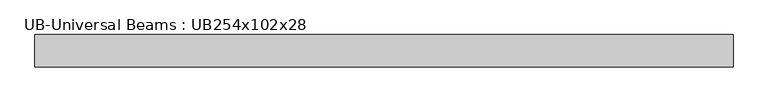
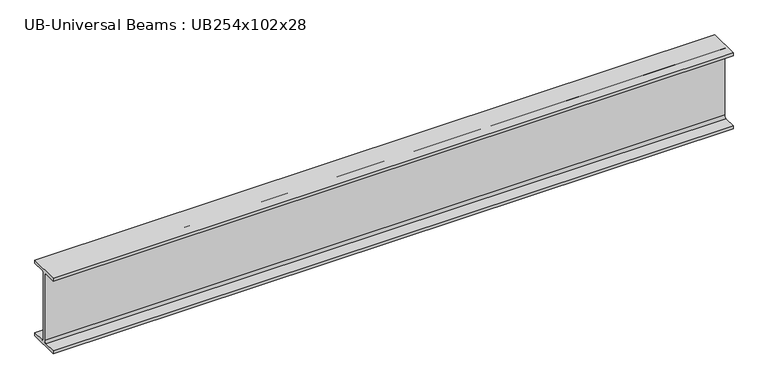
"""IFC4 building model written with IfcOpenShell, lengths in millimetres: beam geometry, UB-Universal Beams : UB254x102x28."""

from ifc_helpers import new_model, si_unit, point, frame, frame_2d, origin, place, context, project, spatial, polyline, circle_curve, trimmed, segment, composite_curve, outline, extrude, source, transform, mapped, element, save


def ub_universal_beams_ub254x102x28_f7ef6108(model_context):
    return source(origin(), model_context, "Body", "SweptSolid", [
        extrude(outline(composite_curve([segment(polyline([(51.1, -120.2), (51.1, -130.2), (-51.1, -130.2), (-51.1, -120.2), (-10.75, -120.2)]), True, "CONTINUOUS"), segment(trimmed(circle_curve(frame_2d((-10.75, -112.6)), 7.6), [point((-10.75, -120.2))], [point((-3.15, -112.6))], True, "CARTESIAN"), True, "CONTINUOUS"), segment(polyline([(-3.15, -112.6), (-3.15, 112.6)]), True, "CONTINUOUS"), segment(trimmed(circle_curve(frame_2d((-10.75, 112.6)), 7.6), [point((-3.15, 112.6))], [point((-10.75, 120.2))], True, "CARTESIAN"), True, "CONTINUOUS"), segment(polyline([(-10.75, 120.2), (-51.1, 120.2), (-51.1, 130.2), (51.1, 130.2), (51.1, 120.2), (10.75, 120.2)]), True, "CONTINUOUS"), segment(trimmed(circle_curve(frame_2d((10.75, 112.6)), 7.6), [point((10.75, 120.2))], [point((3.15, 112.6))], True, "CARTESIAN"), True, "CONTINUOUS"), segment(polyline([(3.15, 112.6), (3.15, -112.6)]), True, "CONTINUOUS"), segment(trimmed(circle_curve(frame_2d((10.75, -112.6)), 7.6), [point((3.15, -112.6))], [point((10.75, -120.2))], True, "CARTESIAN"), True, "CONTINUOUS"), segment(polyline([(10.75, -120.2), (51.1, -120.2)]), True, "CONTINUOUS")], self_intersect=False)), frame((-1171.25, 0.0, 0.0), z_axis=(1.0, 0.0, 0.0), x_axis=(0.0, 1.0, 0.0)), (0.0, 0.0, 1.0), 2215.4),
    ])


if __name__ == "__main__":
    model = new_model("IFC4")
    model_context = context("Model", 3, world=origin())
    ifc_project = project(units=[si_unit("LENGTHUNIT", "METRE", prefix="MILLI")], contexts=[model_context])
    site = spatial("IfcSite", under=ifc_project)
    building = spatial("IfcBuilding", under=site)
    placement = place(None, origin())
    ub_universal_beams_ub254x102x28_shape = ub_universal_beams_ub254x102x28_f7ef6108(model_context)
    element("IfcBeam", 1, ObjectType="UB-Universal Beams : UB254x102x28", at=placement, inside=building, context=model_context, shape_type="MappedRepresentation", body=[
        mapped(ub_universal_beams_ub254x102x28_shape, transform((0.0, 0.0, 0.0), x_axis=(1.0, 0.0, 0.0), y_axis=(0.0, 1.0, 0.0), z_axis=(0.0, 0.0, 1.0))),
    ])
    save(model, "model.ifc")

# Revit data of these elements
# Type "UB-Universal Beams : UB254x102x28"
#   Section Name Key = "UB254X102X28"
#   Width = 10.22 cm
#   Web Thickness = 0.63 cm
#   Web Fillet = 0.76 cm
#   Warping Constant = 28000.0 cm⁶
#   Torsional Moment of Inertia = 9.57 cm⁴
#   Section Area = 36.1 cm²
#   Plastic Modulus weak axis = 54.8 cm³
#   Plastic Modulus strong axis = 353.0 cm³
#   Nominal Weight = 28.2999 kgf/m
#   Moment of Inertia weak axis = 179.00 cm⁴
#   Moment of Inertia strong axis = 4005.00 cm⁴
#   Height = 26.04 cm
#   Flange Thickness = 1.0 cm
#   Elastic Modulus weak axis = 34.9 cm³
#   Elastic Modulus strong axis = 308.0 cm³
#   Centroid Vertical = 13.02 cm
#   Centroid Horizontal = 5.11 cm
#   Bolt Spacing = 5.4 cm
#   Length [instance default] = 4' - 11.05512"
#   Structural Material [instance default] = Metal - Steel 43-275
#   Type Comments = ""
#   Assembly Code = ""
# Element 1 (IfcBeam, "UB-Universal Beams : UB254x102x28")
#   Materials on its faces: "Metal - Steel 43-275"
# Materials
#   "Metal - Steel 43-275": class "Metal", colour RGB 247 247 247, transparency 0, Cost = 0
